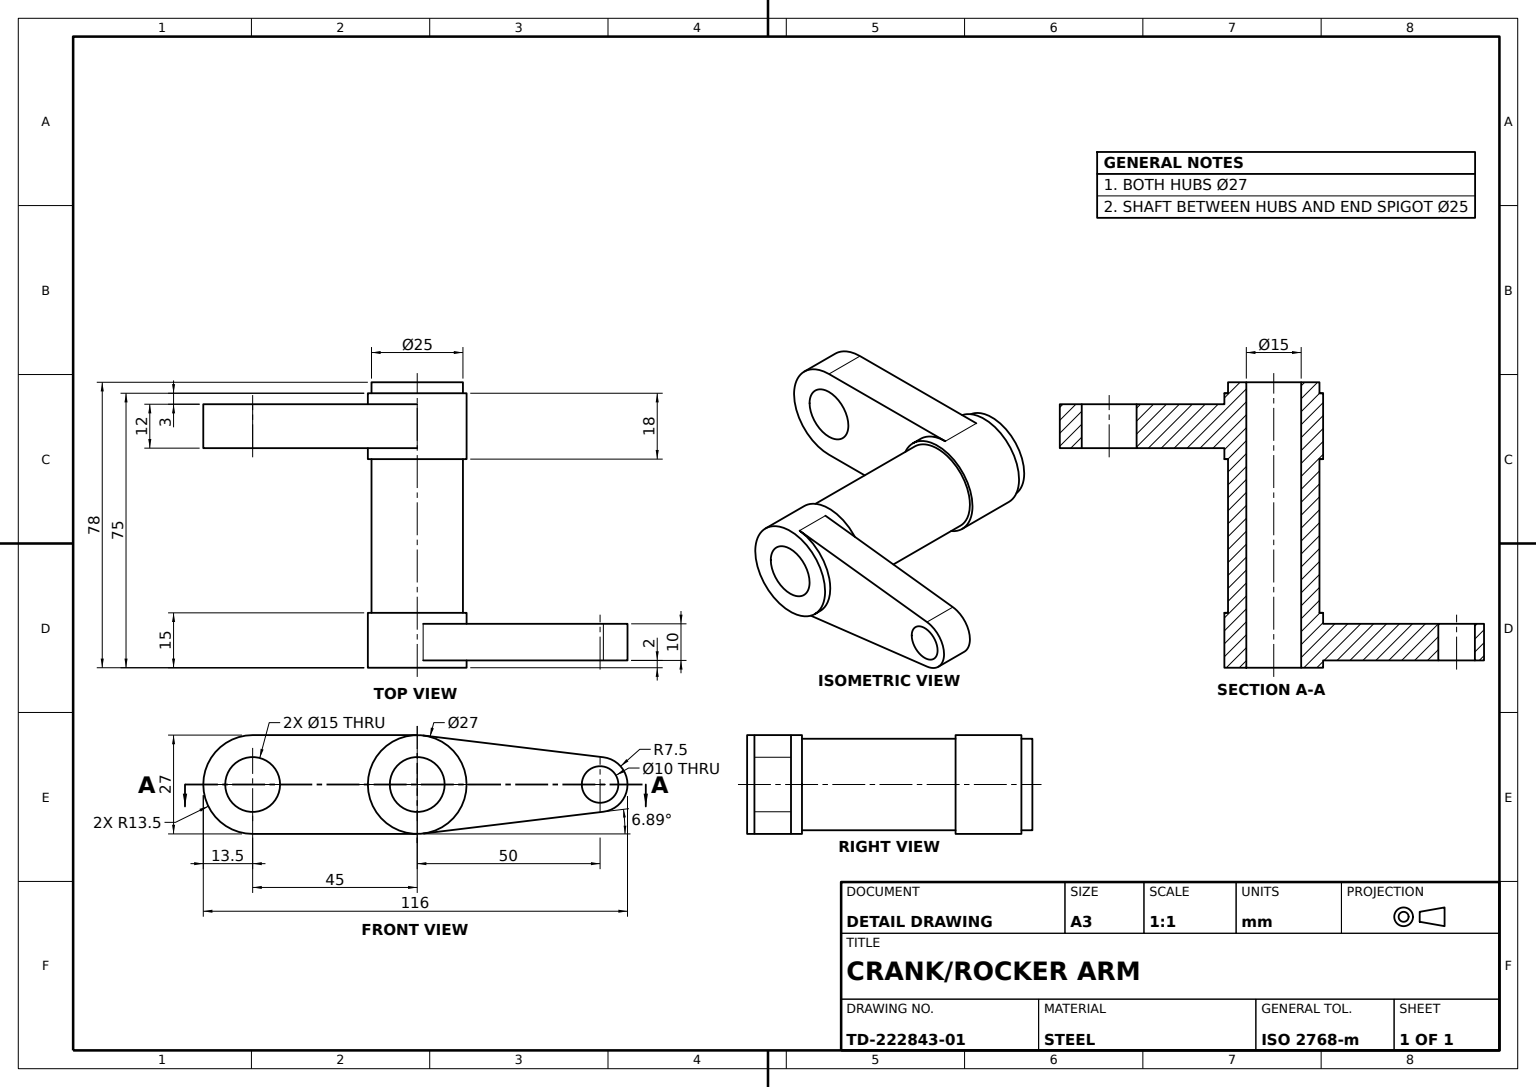
from build123d import *

# Parameters (mm, degrees)
LOWER_ARM_PROFILE_SKETCH_R   = 13.5
LOWER_ARM_PROFILE_SKETCH_R_2 = 7.5
LOWER_CRANK_ARM_DEPTH        = 9
SKETCH1_3_R                  = 7.5
LOWER_ARM_HUB_BOSS_DEPTH     = 6
SHAFT_25_DEPTH               = 75
SHAFT_25_DEPTH_BACK          = 3
SHAFT_25_START               = -9
SHAFT_25_SKETCH_R            = 12.5
SHAFT_25_SKETCH_R_2          = 7.5
SHAFT_COLLAR_SKETCH_R        = 13.5
SHAFT_COLLAR_SKETCH_R_2      = 7.5
SHAFT_COLLAR_DEPTH           = 15
UPPER_START                  = -2
UPPER_ARM_PROFILE_SKETCH_R   = 5
UPPER_CRANK_ARM_DEPTH        = 10


with BuildPart() as part:
    # Lower Arm Profile Sketch → Lower Crank Arm (new, symmetric)
    with BuildSketch(Plane.XY):
        Circle(LOWER_ARM_PROFILE_SKETCH_R)
        Circle(LOWER_ARM_PROFILE_SKETCH_R_2, mode=Mode.SUBTRACT)
    extrude(amount=LOWER_CRANK_ARM_DEPTH, both=True)



with BuildPart() as body_2:
    # Sketch1_3 → Lower Arm Hub Boss (new, symmetric)
    with BuildSketch(Plane.XY):
        with BuildLine():
            ThreePointArc((-45, 13.5), (-58.5, 0), (-45, -13.5))
            Line((-45, -13.5), (0, -13.5))
            ThreePointArc((0, -13.5), (-13.5, 0), (0, 13.5))
            Line((0, 13.5), (-45, 13.5))
        make_face()
        with Locations((-45, 0)):
            Circle(SKETCH1_3_R, mode=Mode.SUBTRACT)
    extrude(amount=LOWER_ARM_HUB_BOSS_DEPTH, both=True)


with BuildPart() as part_1:
    add(part.part)

    add(body_2.part)  # Shaft _25 merges body 2
    # Shaft _25 Sketch → Shaft _25 (add, two sides: drawn at the far end of the back side and taken through both)
    with BuildSketch(Plane.XY.offset(SHAFT_25_START - SHAFT_25_DEPTH_BACK)):
        Circle(SHAFT_25_SKETCH_R)
        Circle(SHAFT_25_SKETCH_R_2, mode=Mode.SUBTRACT)
    extrude(amount=SHAFT_25_DEPTH + SHAFT_25_DEPTH_BACK)

    # Shaft Collar Sketch → Shaft Collar (add)
    with BuildSketch(Plane.XY.offset(66)):
        Circle(SHAFT_COLLAR_SKETCH_R)
        Circle(SHAFT_COLLAR_SKETCH_R_2, mode=Mode.SUBTRACT)
    extrude(amount=-SHAFT_COLLAR_DEPTH)

    # Upper Arm Profile Sketch → Upper Crank Arm (add)
    with BuildSketch(Plane.XY.offset(66).offset(UPPER_START)):
        with BuildLine():
            Line((1.62, 13.402447538), (50.9, 7.445804188))
            ThreePointArc((50.9, 7.445804188), (57.5, 0), (50.9, -7.445804188))
            Line((50.9, -7.445804188), (1.62, -13.402447538))
            ThreePointArc((1.62, -13.402447538), (13.5, 0), (1.62, 13.402447538))
        make_face()
        with Locations((50, 0)):
            Circle(UPPER_ARM_PROFILE_SKETCH_R, mode=Mode.SUBTRACT)
    extrude(amount=-UPPER_CRANK_ARM_DEPTH)


solid = part_1.part
